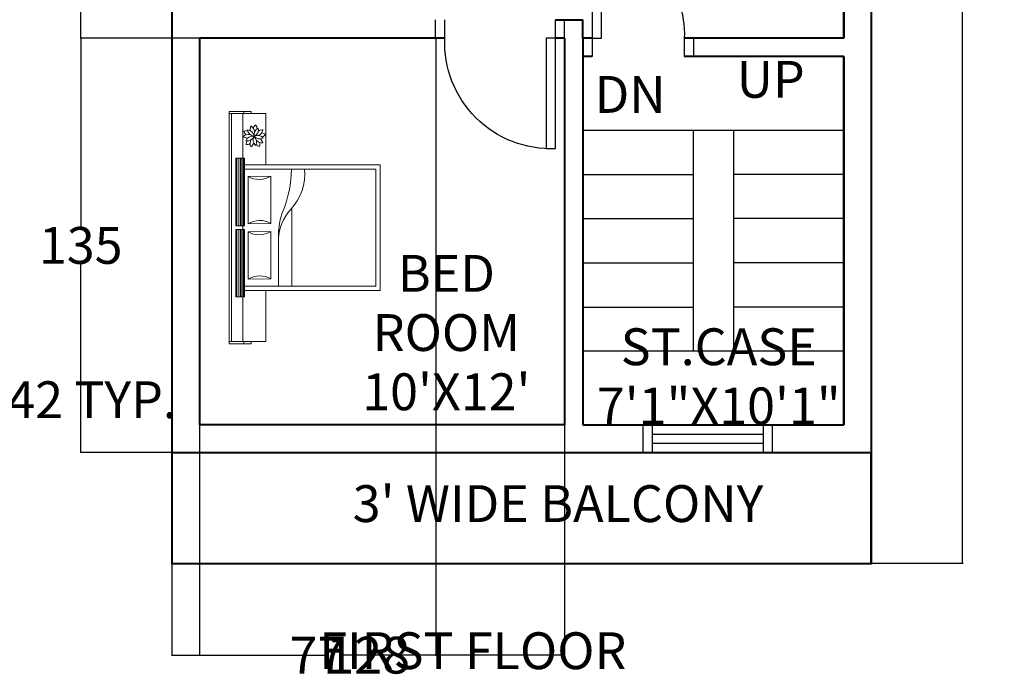
# Model space of a CAD drawing. Units: inches. Extents: x -124 to 612, y -69 to 524.
# Tile 7 of 9: x 287 to 608, y -69 to 146. Entities that reach past the tile are written whole.
import ezdxf
from ezdxf.enums import TextEntityAlignment as Align

# ---------------------------------------------------------------- set-up
doc = ezdxf.new("R2010")
doc.units = ezdxf.units.IN
doc.header["$MEASUREMENT"] = 0
doc.layers.add('5', color=5, linetype='Continuous')
for name, color, linetype, lineweight in [('A-ANNO-DIMS', 2, 'Continuous', 18), ('A-ANNO-TEXT', 1, 'Continuous', 18), ('A-AREA-IDEN', 1, 'Continuous', 18), ('A-DOOR', 4, 'Continuous', 25), ('A-FLOR-HRAL', 8, 'Continuous', 18), ('A-FLOR-STRS', 2, 'Continuous', 25), ('A-FURN', 8, 'Continuous', 18), ('A-GLAZ', 5, 'Continuous', 18), ('A-WALL', 7, 'Continuous', 40)]:
    doc.layers.add(name, color=color, linetype=linetype, lineweight=lineweight)
doc.styles.get("Standard").update_dxf_attribs({"font": 'arial.ttf'})
doc.dimstyles.get("Standard").update_dxf_attribs({"dimtxt": 12, "dimasz": 0.18, "dimexe": 0.18, "dimexo": 0.0625, "dimgap": 0.09, "dimtad": 0, "dimtih": 1, "dimtoh": 1, "dimdec": 0, "dimzin": 0, "dimdsep": 46, "dimlunit": 4, "dimtxsty": 'Standard', "dimcen": 0.09, "dimadec": 0, "dimazin": 0, "dimtfac": 1, "dimtdec": 0, "dimtofl": 0, "dimtmove": 0, "dimatfit": 3, "dimfxl": 1, "dimtolj": 1, "dimtzin": 0, "dimarcsym": 0})

# ---------------------------------------------------------------- blocks, each defined once
blk = doc.blocks.new('V')
at = {"layer": '5'}
for p, q in [((0, 0), (0, 9)), ((3, 9), (39, 9)), ((3, 0), (3, 9)), ((39, 9), (39, 0)), ((42, 9), (42, 0)), ((3, 6), (39, 6)), ((39, 3), (3, 3)), ((39, 0), (3, 0))]:
    blk.add_line(p, q, dxfattribs=at)
blk = doc.blocks.new('A$C7BDD1693')
for p, q in [((0, 2.068), (0, 1.768)), ((0, 2.068), (1.615, 2.068)), ((0.03, 1.768), (0.03, 2.068)), ((0.03, 2.038), (0.64, 2.038)), ((0.64, 2.038), (1.565, 2.038)), ((1.565, 2.038), (1.615, 2.038)), ((1.615, 2.068), (2.54, 2.068)), ((1.615, 2.038), (2.54, 2.038)), ((2.54, 2.068), (3.18, 2.068)), ((3.15, 2.038), (2.54, 2.038)), ((3.15, 1.768), (3.15, 2.068)), ((3.18, 2.068), (3.18, 1.768)), ((0.64, 1.978), (1.565, 1.978)), ((0.64, 1.978), (0.64, 1.858)), ((0.64, 1.963), (1.565, 1.963)), ((0.64, 1.937), (1.565, 1.937)), ((0.64, 1.912), (1.565, 1.912)), ((0.64, 1.893), (1.565, 1.893)), ((1.565, 1.978), (1.565, 1.858)), ((1.615, 1.978), (1.615, 1.858)), ((1.615, 1.978), (2.54, 1.978)), ((1.615, 1.963), (2.54, 1.963)), ((1.615, 1.937), (2.54, 1.937)), ((1.615, 1.912), (2.54, 1.912)), ((1.615, 1.893), (2.54, 1.893)), ((2.54, 1.978), (2.54, 1.858)), ((0.03, 1.868), (0, 1.868)), ((0, 1.768), (0.03, 1.768)), ((0.03, 1.88), (0.64, 1.88)), ((0.03, 1.768), (0.03, 1.568)), ((0.03, 1.768), (0.03, 1.568)), ((0.64, 1.877), (1.565, 1.877)), ((0.64, 1.866), (1.565, 1.866)), ((0.64, 1.858), (1.565, 1.858)), ((0.73, 1.568), (0.73, 1.858)), ((0.79, 1.858), (0.79, 0.06)), ((1.533, 1.81), (0.883, 1.81)), ((0.883, 1.81), (0.887, 1.498)), ((1.537, 1.498), (1.533, 1.81)), ((1.565, 1.88), (1.615, 1.88)), ((1.615, 1.877), (2.54, 1.877)), ((1.615, 1.866), (2.54, 1.866)), ((1.615, 1.858), (2.54, 1.858)), ((2.291, 1.81), (1.641, 1.81)), ((1.641, 1.81), (1.646, 1.498)), ((2.296, 1.498), (2.291, 1.81)), ((2.39, 1.858), (2.39, 0.06)), ((2.45, 1.568), (2.45, 1.858)), ((3.15, 1.88), (2.54, 1.88)), ((3.15, 1.868), (3.18, 1.868)), ((3.15, 1.568), (3.15, 1.768)), ((3.18, 1.768), (3.15, 1.768)), ((0.03, 1.568), (0.73, 1.568)), ((0.73, 1.568), (0.73, 0)), ((0.887, 1.498), (1.537, 1.498)), ((1.646, 1.498), (2.296, 1.498)), ((3.15, 1.568), (2.45, 1.568)), ((2.45, 1.568), (2.45, 0)), ((1.54, 1.392), (0.79, 1.392)), ((1.848, 1.209), (0.79, 1.209)), ((0.73, 0), (2.45, 0)), ((0.79, 0.06), (2.39, 0.06))]:
    blk.add_line(p, q)
for centre, radius, start, end in [((0.626, 1.65), 0.303, 329.8722, 31.8713), ((1.794, 1.658), 0.303, 149.8722, 211.8713), ((1.384, 1.65), 0.303, 329.8722, 31.8713), ((2.553, 1.658), 0.303, 149.8722, 211.8713), ((2.74, 1.667), 0.115, 63.1324, 112.6013), ((2.798, 1.845), 0.125, 215.1301, 245.4931), ((2.879, 1.849), 0.155, 184.2105, 205.3514), ((2.726, 1.74), 0.0968, 57.5086, 91.2476), ((2.884, 1.823), 0.106, 170.7761, 244.5159), ((2.743, 1.749), 0.098, 347.0447, 68.2473), ((2.938, 1.802), 0.125, 143.1301, 173.4932), ((2.751, 1.802), 0.115, 351.1324, 40.6013), ((2.944, 1.713), 0.106, 98.7761, 172.5159), ((2.83, 1.825), 0.098, 275.0447, 356.2473), ((2.967, 1.726), 0.155, 112.2105, 133.3514), ((2.883, 1.833), 0.115, 279.1324, 328.6013), ((2.817, 1.838), 0.0968, 345.5086, 19.2476), ((2.941, 1.655), 0.125, 71.1301, 101.4931), ((2.791, 1.624), 0.0968, 129.5086, 163.2476), ((2.735, 1.803), 0.155, 256.2105, 277.3514), ((2.788, 1.643), 0.098, 59.0447, 140.2473), ((2.761, 1.8), 0.106, 242.7761, 316.5159), ((2.865, 1.615), 0.115, 135.1324, 184.6013), ((2.713, 1.725), 0.125, 287.1301, 317.4932), ((2.903, 1.653), 0.098, 131.0447, 212.2473), ((2.745, 1.676), 0.106, 314.7761, 28.5159), ((2.858, 1.622), 0.106, 26.7761, 100.5159), ((2.929, 1.765), 0.098, 203.0447, 284.2473), ((2.953, 1.718), 0.115, 207.1324, 256.6013), ((2.734, 1.652), 0.155, 328.2105, 349.3514), ((2.802, 1.607), 0.125, 359.1301, 29.4932), ((2.937, 1.782), 0.0968, 273.5086, 307.2476), ((2.877, 1.605), 0.155, 40.2105, 61.3514), ((2.921, 1.65), 0.0968, 201.5086, 235.2476)]:
    blk.add_arc(centre, radius, start, end)
for centre, major_axis, ratio, start_param, end_param in [((1.413, 0.552), (0, -0.842), 0.84, 2.512571, 3.097265), ((1.474, 0.023), (0, -1.371), 0.84, 2.845884, 3.083884), ((2.394, 3.329), (0, -2.112), 0.84, -0.336035, -0.002349), ((2.261, 1.856), (0.259, -0.793), 0.868451, -0.988378, -0.183496)]:
    blk.add_ellipse(centre, major_axis=major_axis, ratio=ratio, start_param=start_param, end_param=end_param)
blk = doc.blocks.new('DOOR-36IN-SINGLE')
for p, q in [((0, 6), (0, 0)), ((3, 6), (3, 0)), ((39, 6), (39, 0)), ((42, 6), (42, 0))]:
    blk.add_line(p, q)
blk.add_lwpolyline([(39, 6), (36, 6), (36, 42), (39, 42)], close=True)
blk.add_arc((37.5, 7.5), 34.53, 87.5104, 182.4896)
blk = doc.blocks.new('DOOR-30IN-STAIR')
for p, q in [((0, 30.04), (0, 36.04)), ((3, 30.04), (3, 36.04)), ((33, 30.04), (33, 36.04)), ((36, 30.04), (36, 36.04))]:
    blk.add_line(p, q)
blk.add_lwpolyline([(3, 30.04), (6, 30.04), (6, 0.04), (3, 0.04)], close=True)
blk.add_arc((4.5, 28.54), 28.54, 266.9872, 3.0128)
blk = doc.blocks.new('STAIR-FLIGHT-36IN')
for p, q in [((36, 0), (36, 72)), ((0, 57.6), (36, 57.6)), ((0, 43.2), (36, 43.2)), ((0, 28.8), (36, 28.8)), ((0, 14.4), (36, 14.4))]:
    blk.add_line(p, q)
blk = doc.blocks.new('*D35')
at = {"layer": 'A-ANNO-DIMS', "color": 0, "lineweight": -2, "transparency": 16777216}
for p, q in [((164.01, 16.09), (164.01, 22.51)), ((206.01, 16.09), (206.01, 22.51)), ((164.19, 22.33), (205.83, 22.33)), ((206.01, 22.33), (206.19, 22.33))]:
    blk.add_line(p, q, dxfattribs=at)
at = {"layer": 'A-ANNO-DIMS', "color": 0, "transparency": 16777216}
for points in [[(164.19, 22.36), (164.19, 22.3), (164.01, 22.33)], [(205.83, 22.36), (205.83, 22.3), (206.01, 22.33)]]:
    blk.add_solid(points, dxfattribs=at)
at = {"layer": 'Defpoints', "color": 0, "transparency": 16777216}
for p in [(206.01, 22.33), (164.01, 16.03), (206.01, 16.03)]:
    blk.add_point(p, dxfattribs=at)
at = {"layer": 'A-ANNO-DIMS', "color": 0, "transparency": 16777216, "insert": (274.84, 22.33), "char_height": 12, "attachment_point": 5}
blk.add_mtext('\\A1;WINDOW 42 TYP.', dxfattribs=at)
blk = doc.blocks.new('*D50')
at = {"layer": 'A-ANNO-DIMS', "color": 0, "lineweight": -2, "transparency": 16777216}
for p, q in [((565.08, 485.1), (594.85, 485.1)), ((594.67, 484.92), (594.67, 233.32)), ((594.67, -30.72), (594.67, 220.89)), ((564.78, -30.9), (594.85, -30.9))]:
    blk.add_line(p, q, dxfattribs=at)
at = {"layer": 'A-ANNO-DIMS', "color": 0, "transparency": 16777216}
for points in [[(594.64, 484.92), (594.7, 484.92), (594.67, 485.1)], [(594.64, -30.72), (594.7, -30.72), (594.67, -30.9)]]:
    blk.add_solid(points, dxfattribs=at)
at = {"layer": 'Defpoints', "color": 0, "transparency": 16777216}
for p in [(565.02, 485.1), (594.67, 485.1), (564.72, -30.9)]:
    blk.add_point(p, dxfattribs=at)
at = {"layer": 'A-ANNO-DIMS', "color": 0, "transparency": 16777216, "insert": (594.67, 227.1), "char_height": 12, "attachment_point": 5}
blk.add_mtext('\\A1;516', dxfattribs=at)
blk = doc.blocks.new('*D54')
at = {"layer": 'A-ANNO-DIMS', "color": 0, "lineweight": -2, "transparency": 16777216}
for p, q in [((346.02, 140.04), (346.02, -61.03)), ((423.02, 140.04), (423.02, -61.03)), ((346.2, -60.85), (375.88, -60.85)), ((422.84, -60.85), (393.15, -60.85))]:
    blk.add_line(p, q, dxfattribs=at)
at = {"layer": 'A-ANNO-DIMS', "color": 0, "transparency": 16777216}
for points in [[(346.2, -60.82), (346.2, -60.88), (346.02, -60.85)], [(422.84, -60.82), (422.84, -60.88), (423.02, -60.85)]]:
    blk.add_solid(points, dxfattribs=at)
at = {"layer": 'Defpoints', "color": 0, "transparency": 16777216}
for p in [(346.02, 140.1), (423.02, 140.1), (423.02, -60.85)]:
    blk.add_point(p, dxfattribs=at)
at = {"layer": 'A-ANNO-DIMS', "color": 0, "transparency": 16777216, "insert": (384.52, -60.85), "char_height": 12, "attachment_point": 5}
blk.add_mtext('\\A1;77', dxfattribs=at)
blk = doc.blocks.new('*D58')
at = {"layer": 'A-ANNO-DIMS', "color": 0, "lineweight": -2, "transparency": 16777216}
for p, q in [((345.95, 140.1), (307.19, 140.1)), ((307.37, 139.92), (307.37, 78.83)), ((307.37, 5.28), (307.37, 66.38)), ((336.95, 5.1), (307.19, 5.1))]:
    blk.add_line(p, q, dxfattribs=at)
at = {"layer": 'A-ANNO-DIMS', "color": 0, "transparency": 16777216}
for points in [[(307.34, 139.92), (307.4, 139.92), (307.37, 140.1)], [(307.34, 5.28), (307.4, 5.28), (307.37, 5.1)]]:
    blk.add_solid(points, dxfattribs=at)
at = {"layer": 'Defpoints', "color": 0, "transparency": 16777216}
for p in [(307.37, 140.1), (346.02, 140.1), (337.02, 5.1)]:
    blk.add_point(p, dxfattribs=at)
at = {"layer": 'A-ANNO-DIMS', "color": 0, "transparency": 16777216, "insert": (307.37, 72.6), "char_height": 12, "attachment_point": 5}
blk.add_mtext('\\A1;135', dxfattribs=at)
blk = doc.blocks.new('*D68')
at = {"layer": 'A-ANNO-DIMS', "color": 0, "lineweight": -2, "transparency": 16777216}
for p, q in [((465.02, 14.04), (465.02, -61.03)), ((337.02, 5.04), (337.02, -61.03)), ((337.2, -60.85), (388.22, -60.85)), ((464.84, -60.85), (413.81, -60.85))]:
    blk.add_line(p, q, dxfattribs=at)
at = {"layer": 'A-ANNO-DIMS', "color": 0, "transparency": 16777216}
for points in [[(337.2, -60.82), (337.2, -60.88), (337.02, -60.85)], [(464.84, -60.82), (464.84, -60.88), (465.02, -60.85)]]:
    blk.add_solid(points, dxfattribs=at)
at = {"layer": 'Defpoints', "color": 0, "transparency": 16777216}
for p in [(465.02, 14.1), (337.02, 5.1), (465.02, -60.85)]:
    blk.add_point(p, dxfattribs=at)
at = {"layer": 'A-ANNO-DIMS', "color": 0, "transparency": 16777216, "insert": (401.02, -60.85), "char_height": 12, "attachment_point": 5}
blk.add_mtext('\\A1;128', dxfattribs=at)
blk = doc.blocks.new('*D69')
at = {"layer": 'A-ANNO-DIMS', "color": 0, "lineweight": -2, "transparency": 16777216}
for p, q in [((345.95, 212.1), (307.19, 212.1)), ((307.37, 211.92), (307.37, 182.22)), ((307.37, 140.28), (307.37, 169.99)), ((345.95, 140.1), (307.19, 140.1))]:
    blk.add_line(p, q, dxfattribs=at)
at = {"layer": 'A-ANNO-DIMS', "color": 0, "transparency": 16777216}
for points in [[(307.34, 211.92), (307.4, 211.92), (307.37, 212.1)], [(307.34, 140.28), (307.4, 140.28), (307.37, 140.1)]]:
    blk.add_solid(points, dxfattribs=at)
at = {"layer": 'Defpoints', "color": 0, "transparency": 16777216}
for p in [(307.37, 212.1), (346.02, 212.1), (346.02, 140.1)]:
    blk.add_point(p, dxfattribs=at)
at = {"layer": 'A-ANNO-DIMS', "color": 0, "transparency": 16777216, "insert": (307.37, 176.1), "char_height": 12, "attachment_point": 5}
blk.add_mtext('\\A1;72', dxfattribs=at)

msp = doc.modelspace()

# ---------------------------------------------------------------- linework, layer by layer
at = {"layer": 'A-FLOR-HRAL'}
for p, q in [((337.3169, 5.1047), (337.3169, -30.8953)), ((564.7169, -30.8953), (564.7169, 5.1047)), ((337.0169, -31.1953), (565.0169, -31.1953)), ((337.3169, -30.8953), (564.7169, -30.8953))]:
    msp.add_line(p, q, dxfattribs=at)
at = {"layer": 'A-FLOR-STRS'}
for p, q in [((471.0169, 110.1047), (556.0169, 110.1047)), ((556.0169, 38.1047), (471.0169, 38.1047))]:
    msp.add_line(p, q, dxfattribs=at)
msp.add_lwpolyline([(471.0169, 119.2102, 0, 0, 0), (538.1149, 119.2102, 0, 0, 0), (538.1149, 66.9047, 12, 0, 0), (538.1149, 38.1047, 0, 0, 0)], format="xyseb", dxfattribs=at)
at = {"layer": 'A-WALL'}
for p, q in [((337.0169, 485.1047), (337.0169, -31.1953)), ((565.0169, -31.1953), (565.0169, 485.1047)), ((556.0169, 140.1047), (556.0169, 188.1047)), ((556.0169, 188.1047), (556.0169, 140.1047)), ((462.0169, 146.1047), (471.0169, 146.1047)), ((471.0169, 140.1047), (471.0169, 146.1047)), ((426.0169, 140.1047), (346.0169, 140.1047)), ((346.0169, 140.1047), (346.0169, 14.1047)), ((426.0169, 140.1047), (346.0169, 140.1047)), ((465.0169, 140.1047), (462.0169, 140.1047)), ((465.0169, 140.1047), (465.0169, 14.1047)), ((471.0169, 140.1047), (471.0169, 14.1047)), ((474.0169, 140.1047), (471.0169, 140.1047)), ((556.0169, 140.1047), (504.0169, 140.1047)), ((474.0169, 134.1047), (471.0169, 134.1047)), ((556.0169, 134.1047), (504.0169, 134.1047)), ((556.0169, 14.1047), (556.0169, 134.1047)), ((556.0169, 134.1047), (556.0169, 14.1047)), ((465.0169, 14.1047), (346.0169, 14.1047)), ((471.0169, 14.1047), (556.0169, 14.1047)), ((337.0169, 5.1047), (565.0169, 5.1047))]:
    msp.add_line(p, q, dxfattribs=at)

# ---------------------------------------------------------------- block references
at = {"layer": 'A-DOOR', "extrusion": (0, 0, -1), "zscale": -1, "rotation": 180}
for name, p in [('DOOR-30IN-STAIR', (-471.0166, 170.1437)), ('DOOR-36IN-SINGLE', (-423.0166, 146.1047))]:
    msp.add_blockref(name, p, dxfattribs=at)
at = {"layer": 'A-FLOR-STRS'}
msp.add_blockref('STAIR-FLIGHT-36IN', (471.0166, 38.1046), dxfattribs=at)
at = {"layer": 'A-FLOR-STRS', "rotation": 180}
msp.add_blockref('STAIR-FLIGHT-36IN', (556.0172, 110.1047), dxfattribs=at)
at = {"layer": 'A-FURN', "xscale": 23.78825355168716, "yscale": 23.78825355168716, "zscale": 23.78825355168716, "rotation": 90}
msp.add_blockref('A$C7BDD1693', (404.9425, 40.5777), dxfattribs=at)
at = {"layer": 'A-GLAZ'}
msp.add_blockref('V', (490.6773, 5.1047), dxfattribs=at)

# ---------------------------------------------------------------- texts
at = {"layer": 'A-ANNO-TEXT'}
for s, p in [('UP', (532.1698, 120.6825)), ('DN', (486.391, 115.7709)), ('FIRST FLOOR', (435.122, -65.4171))]:
    msp.add_text(s, height=12, dxfattribs=at).set_placement(p, align=Align.CENTER)
at = {"layer": 'A-AREA-IDEN'}
for s, p in [('BED', (426.5042, 57.4814)), ('ROOM', (426.5042, 38.2044)), ('ST.CASE', (515.2613, 33.5845)), ("10'X12'", (426.5042, 18.9275)), ('7\'1"X10\'1"', (515.2613, 14.3076)), ("3' WIDE BALCONY", (462.8796, -17.5037))]:
    msp.add_text(s, height=12, dxfattribs=at).set_placement(p, align=Align.CENTER)

# ---------------------------------------------------------------- dimensions: what is measured, and where the dimension line sits
at = {"layer": 'A-ANNO-DIMS'}
for base, p1, p2, picture, middle in [((594.6669, 485.1047), (564.7169, -30.8953), (565.0169, 485.1047), '*D50', (594.6669, 227.1047)), ((307.3669, 212.1047), (346.0169, 140.1047), (346.0169, 212.1047), '*D69', (307.3669, 176.1047)), ((307.3669, 140.1047), (337.0169, 5.1047), (346.0169, 140.1047), '*D58', (307.3669, 72.6047))]:
    dim = msp.add_linear_dim(base=base, p1=p1, p2=p2, angle=90, dimstyle='Standard', override={"dimdec": 0, "dimlfac": 1, "dimrnd": 0, "dimzin": 0, "dimdsep": 46, "dimlunit": 2}, dxfattribs=at)
    dim.commit()
    dim.dimension.update_dxf_attribs({"geometry": picture, "text_midpoint": middle})
for base, p1, p2, picture, middle in [((423.0169, -60.8453), (346.0169, 140.1047), (423.0169, 140.1047), '*D54', (384.5169, -60.8453)), ((465.0169, -60.8453), (337.0169, 5.1047), (465.0169, 14.1047), '*D68', (401.0169, -60.8453))]:
    dim = msp.add_linear_dim(base=base, p1=p1, p2=p2, dimstyle='Standard', override={"dimdec": 0, "dimlfac": 1, "dimrnd": 0, "dimzin": 0, "dimdsep": 46, "dimlunit": 2}, dxfattribs=at)
    dim.commit()
    dim.dimension.update_dxf_attribs({"geometry": picture, "text_midpoint": middle})
dim = msp.add_linear_dim(base=(206.0117, 22.3291), p1=(164.0117, 16.0291), p2=(206.0117, 16.0291), text='WINDOW <> TYP.', dimstyle='Standard', override={"dimdec": 0, "dimlfac": 1, "dimrnd": 0, "dimzin": 0, "dimdsep": 46, "dimlunit": 2}, dxfattribs=at)
dim.commit()
dim.dimension.update_dxf_attribs({"geometry": '*D35', "text_midpoint": (274.8397, 22.3291)})

doc.saveas('drawing.dxf')
